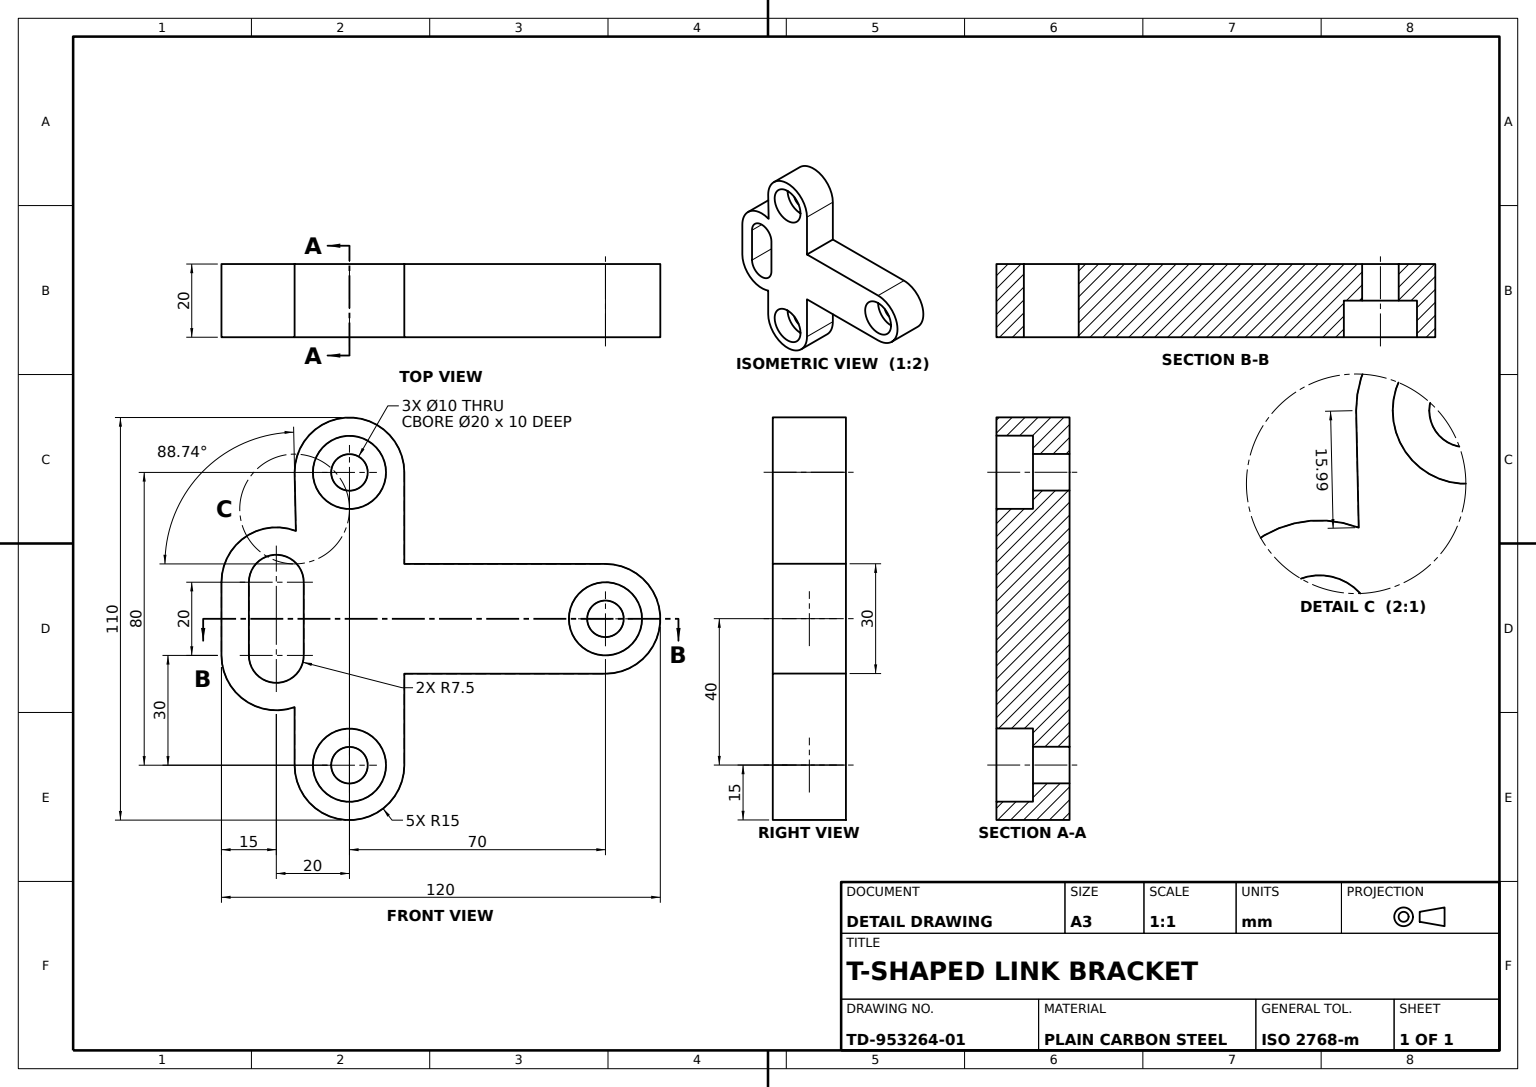
SolidWorks part; units mm, degrees
material "Plain Carbon Steel"
ref_plane "Front Plane" through (0, 0, 0) normal (0, 0, 1) x (1, 0, 0)
ref_plane "Top Plane" through (0, 0, 0) normal (0, 1, 0) x (1, 0, 0)
ref_plane "Right Plane" through (0, 0, 0) normal (1, 0, 0) x (0, 0, -1)
sketch "T Profile Sketch" plane through (0, 0, 0) normal (0, 0, 1) x (1, 0, 0)
  line L4 (-35, 10) -> (-35, -10)
  line L5 (-27.5, 10) -> (-27.5, -10)
  line L6 (-15, 40) -> (-14.6477, 24.0126)
  line L7 (-15, -40) -> (-15, -24.1421)
  line L8 (-12.5, 10) -> (-12.5, -10)
  line L9 (70, 15) -> (15, 15)
  line L10 (15, 15) -> (15, 40)
  line L11 (70, -15) -> (15, -15)
  line L12 (15, -15) -> (15, -40)
  arc A1 (15, 40) -> (-14.9854, 39.3392) centre (0, 40) ccw
  arc A2 (-15, -40) -> (15, -40) centre (0, -40) ccw
  arc A3 (70, -15) -> (70, 15) centre (70, 0) ccw
  arc A5 (-14.6477, 24.0126) -> (-35, 10) centre (-20, 10) ccw
  arc A6 (-35, -10) -> (-15, -24.1421) centre (-20, -10) ccw
  arc A7 (-12.5, 10) -> (-27.5, 10) centre (-20, 10) ccw
  arc A8 (-27.5, -10) -> (-12.5, -10) centre (-20, -10) ccw
  dimension "D1" = 30
  dimension "D2" = 30
  dimension "D3" = 30
  dimension "D4" = 30
  dimension "D5" = 30
  dimension "D6" = 30
  dimension "D7" = 15
  dimension "D8" = 80
  dimension "D9" = 40
  dimension "D10" = 70
  dimension "D11" = 20
  dimension "D12" = 10
  dimension "D13" = 20
  dimension "D14" = 15.9913
extrude "T Bracket Plate 20mm" add sketch "T Profile Sketch" along normal blind 20 contours L4 A6 L7 A2 L12 L11 A3 L9 L10 A1 L6 A5 A8 L5 A7 L8
sketch "Pocket A Sketch" plane through (0, 0, 20) normal (0, 0, 1) x (1, 0, 0)
  circle A0 centre (0, 40) radius 10
  circle A1 centre (0, -40) radius 10
  circle A2 centre (70, 0) radius 10
  dimension "D1" = 20
extrude "Triangular Pocket A 10mm" cut sketch "Pocket A Sketch" against normal blind 10
sketch "Pocket B Sketch" plane through (0, 0, 10) normal (0, 0, 1) x (1, 0, 0)
  circle A0 centre (0, 40) radius 5
  circle A1 centre (0, -40) radius 5
  circle A2 centre (70, 0) radius 5
  dimension "D1" = 10
extrude "Triangular Pocket B 10mm" cut sketch "Pocket B Sketch" against normal blind 10
